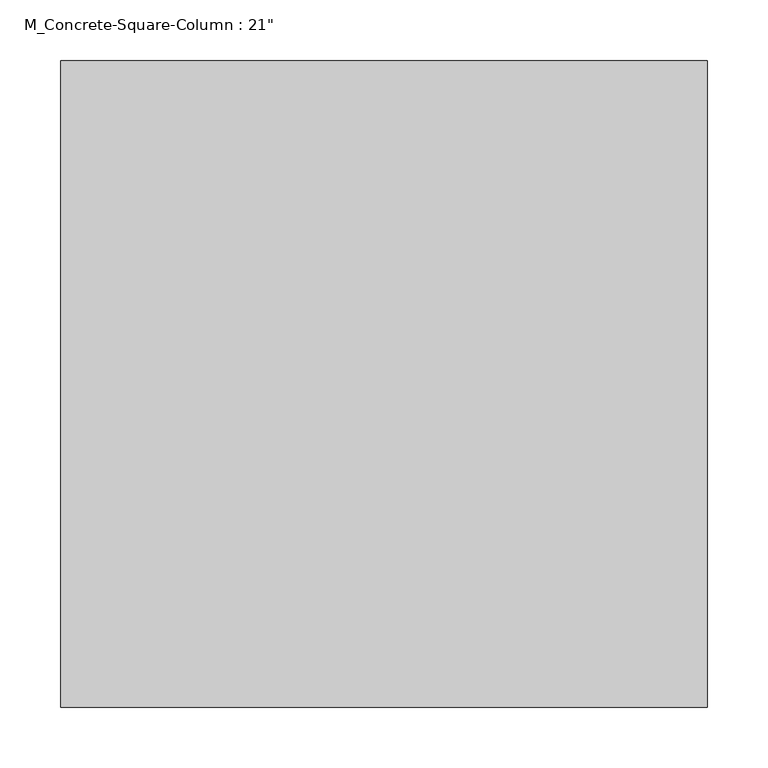
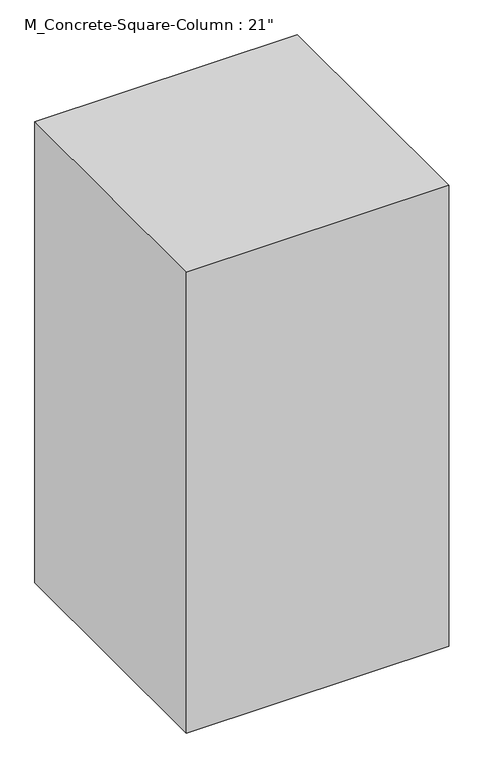
"""IFC4 building model written with IfcOpenShell, lengths in millimetres: column geometry."""

from ifc_helpers import new_model, si_unit, frame, origin, place, context, project, spatial, polyline, outline, extrude, source, transform, mapped, element, save


def column_66439ef4(model_context):
    return source(origin(), model_context, "Body", "SweptSolid", [
        extrude(outline(polyline([(266.7, 266.7), (266.7, -266.7), (-266.7, -266.7), (-266.7, 266.7), (266.7, 266.7)])), frame((0.0, 0.0, -2133.6), z_axis=(0.0, 0.0, 1.0), x_axis=(1.0, 0.0, 0.0)), (0.0, 0.0, 1.0), 990.6),
    ])


if __name__ == "__main__":
    model = new_model("IFC4")
    model_context = context("Model", 3, world=origin())
    ifc_project = project(units=[si_unit("LENGTHUNIT", "METRE", prefix="MILLI")], contexts=[model_context])
    site = spatial("IfcSite", under=ifc_project)
    building = spatial("IfcBuilding", under=site)
    placement = place(None, origin())
    column_shape = column_66439ef4(model_context)
    element("IfcColumn", 1, ObjectType="M_Concrete-Square-Column : 21\"", at=placement, inside=building, context=model_context, shape_type="MappedRepresentation", body=[
        mapped(column_shape, transform((0.0, 0.0, 0.0), x_axis=(1.0, 0.0, 0.0), y_axis=(0.0, 1.0, 0.0), z_axis=(0.0, 0.0, 1.0))),
    ])
    save(model, "model.ifc")

# Revit data of these elements
# Type "M_Concrete-Square-Column : 21\""
#   b = 533.4 mm
#   Structural Material [instance default] = Concrete, Cast-in-Place gray
# Element 1 (IfcColumn, "M_Concrete-Square-Column : 21\"")
#   Materials on its faces: "Concrete, Cast-in-Place gray"
# Materials
#   "Concrete, Cast-in-Place gray": class "Concrete", colour RGB 192 192 192, transparency 0, Description = "Cast-in-place concrete", Cost = 0
